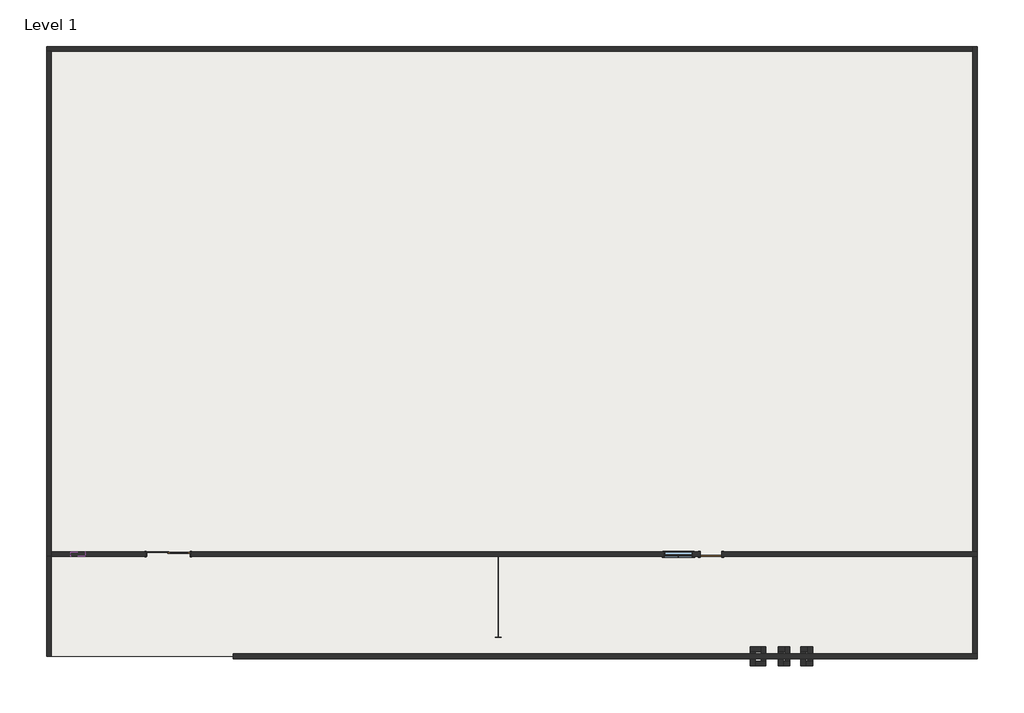
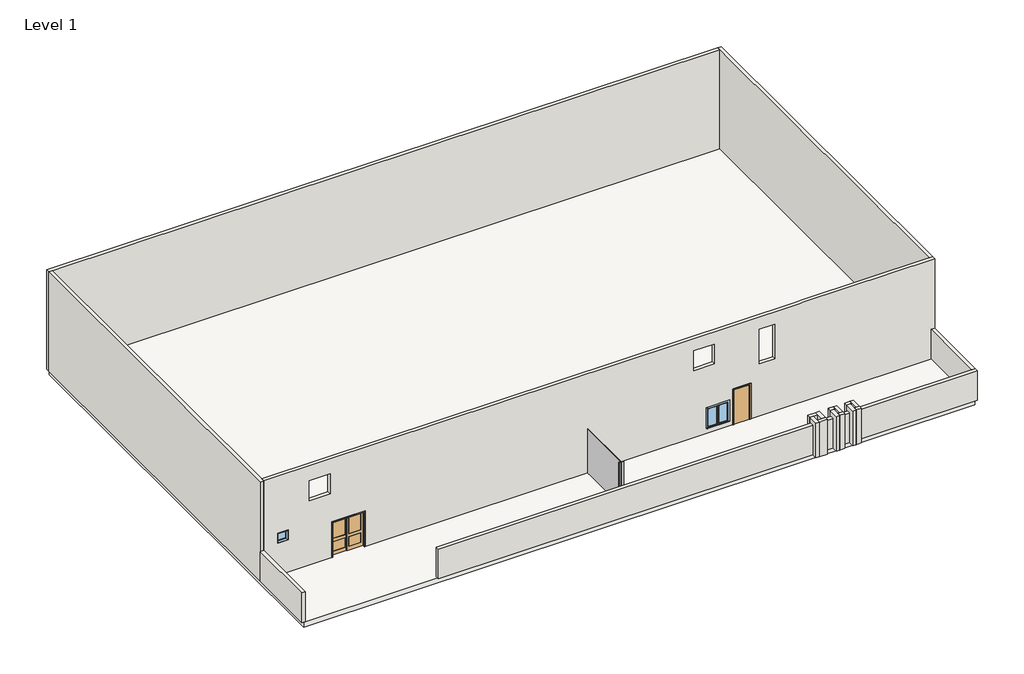
# One storey: 19 walls, 2 doors, 2 windows, 1 column, 1 slab.
"""IFC4 building model written with IfcOpenShell, lengths in millimetres."""

from ifc_helpers import new_model, si_unit, frame, origin, origin_with_axes, place, context, project, spatial, polyline, outline, extrude, faceted_brep, transform, mapped, element, save
from components import w_shapes_column_w10x49_8dea7e6f, door_6868039c, door_54dd4da4, window_0862ab64, window_6846e476

model = new_model("IFC4")

# Units and contexts
model_context = context("Model", 3, world=origin())
ifc_project = project(units=[si_unit("LENGTHUNIT", "METRE", prefix="MILLI")], contexts=[model_context])

# Site, building, storey
site = spatial("IfcSite", under=ifc_project)
building = spatial("IfcBuilding", under=site)
storey = spatial("IfcBuildingStorey", under=building, Name="Level 1", Elevation=0.0)

# Column
placement = place(None, origin())
w_shapes_column_w10x49_shape = w_shapes_column_w10x49_8dea7e6f(model_context)
element("IfcColumn", 1, ObjectType="W Shapes-Column : W10X49", at=placement, inside=storey, context=model_context, shape_type="MappedRepresentation", body=[
    mapped(w_shapes_column_w10x49_shape, transform((-3499.1858676, -16576.9422847, 0.0), x_axis=(1.0, 0.0, 0.0), y_axis=(0.0, 1.0, 0.0), z_axis=(0.0, 0.0, 1.0))),
])

# Doors
door_shape = door_6868039c(model_context)
element("IfcDoor", 2, ObjectType="Door-Interior-Double-Sliding-2_Panel-Wood : 72\" x 84\"", at=placement, inside=storey, context=model_context, shape_type="MappedRepresentation", body=[
    mapped(door_shape, transform((-17399.3252602, -14815.695124, 0.0), x_axis=(1.0, 0.0, 0.0), y_axis=(0.0, 1.0, 0.0), z_axis=(0.0, 0.0, 1.0))),
])
door_2_shape = door_54dd4da4(model_context)
element("IfcDoor", 3, ObjectType="Single-Flush : 36\" x 84\"", at=placement, inside=storey, context=model_context, shape_type="MappedRepresentation", body=[
    mapped(door_2_shape, transform((5460.6747398, -14818.870124, 0.0), x_axis=(-1.0, 0.0, 0.0), y_axis=(0.0, -1.0, 0.0), z_axis=(0.0, 0.0, 1.0))),
])

# Slab
element("IfcSlab", 4, ObjectType="Generic - 12\"", at=placement, inside=storey, context=model_context, shape_type="SweptSolid", body=[
    extrude(outline(polyline([(16585.8747398, 6480.1537948), (16585.8747398, -19123.0462052), (-22428.5252602, -19123.0462052), (-22428.5252602, 6480.1537948), (16585.8747398, 6480.1537948)])), frame((0.0, 0.0, -304.8), z_axis=(0.0, 0.0, 1.0), x_axis=(1.0, 0.0, 0.0)), (0.0, 0.0, 1.0), 304.8),
])

# Walls
element("IfcWall", 5, ObjectType="Generic - 8\"", at=placement, inside=storey, context=model_context, shape_type="Brep", body=[
    faceted_brep([(-22530.1252602, 6378.5537948, 0.0), (-22326.9252602, 6378.5537948, 0.0), (16484.2747398, 6378.5537948, 0.0), (16484.2747398, 6378.5537948, 6096.0), (-22326.9252602, 6378.5537948, 6096.0), (-22530.1252602, 6378.5537948, 6096.0), (-22530.1252602, 6581.7537948, 0.0), (-22530.1252602, 6581.7537948, 6096.0), (16484.2747398, 6581.7537948, 6096.0), (16484.2747398, 6581.7537948, 0.0)], [[[0, 1, 2, 3, 4, 5]], [[6, 7, 8, 9]], [[2, 1, 0, 6, 9]], [[5, 4, 3, 8, 7]], [[0, 5, 7, 6]], [[3, 2, 9, 8]]]),
])
element("IfcWall", 6, ObjectType="Generic - 8\"", at=placement, inside=storey, context=model_context, shape_type="Brep", body=[
    faceted_brep([(-22326.9252602, -14920.470124, 6096.0), (-22326.9252602, -14920.470124, 1828.8), (-22326.9252602, -14920.470124, 0.0), (-22326.9252602, -14717.270124, 0.0), (-22326.9252602, 6378.5537948, 0.0), (-22326.9252602, 6378.5537948, 6096.0), (-22326.9252602, -14717.270124, 6096.0), (-22530.1252602, -14920.470124, 0.0), (-22530.1252602, -14920.470124, 1828.8), (-22530.1252602, -14920.470124, 6096.0), (-22530.1252602, 6378.5537948, 6096.0), (-22530.1252602, 6378.5537948, 0.0)], [[[0, 1, 2, 3, 4, 5, 6]], [[7, 8, 9, 10, 11]], [[4, 3, 2, 7, 11]], [[0, 6, 5, 10, 9]], [[5, 4, 11, 10]], [[0, 9, 8, 7, 2, 1]]]),
])
element("IfcWall", 7, ObjectType="Generic - 8\"", at=placement, inside=storey, context=model_context, shape_type="Brep", body=[
    faceted_brep([(-22326.9252602, -14717.270124, 6096.0), (8806.3760973, -14717.270124, 6096.0), (9009.5760973, -14717.270124, 6096.0), (16484.2747398, -14717.270124, 6096.0), (16687.4747398, -14717.270124, 6096.0), (16687.4747398, -14717.270124, 0.0), (16484.2747398, -14717.270124, 0.0), (5917.8747398, -14717.270124, 0.0), (5917.8747398, -14717.270124, 2133.6), (5003.4747398, -14717.270124, 2133.6), (5003.4747398, -14717.270124, 0.0), (-16459.5252602, -14717.270124, 0.0), (-16459.5252602, -14717.270124, 2159.0), (-18339.1252602, -14717.270124, 2159.0), (-18339.1252602, -14717.270124, 0.0), (-22326.9252602, -14717.270124, 0.0), (-19685.3252602, -14717.270124, 5185.1493756), (-19685.3252602, -14717.270124, 3965.9493756), (-18466.1252602, -14717.270124, 3965.9493756), (-18466.1252602, -14717.270124, 5185.1493756), (-20904.5252602, -14717.270124, 1976.5444437), (-20904.5252602, -14717.270124, 2586.1444437), (-21514.1252602, -14717.270124, 2586.1444437), (-21514.1252602, -14717.270124, 1976.5444437), (6476.6747398, -14717.270124, 3200.4), (7391.0747398, -14717.270124, 3200.4), (7391.0747398, -14717.270124, 5334.0), (6476.6747398, -14717.270124, 5334.0), (2666.6747398, -14717.270124, 5334.0), (2666.6747398, -14717.270124, 4114.8), (3885.8747398, -14717.270124, 4114.8), (3885.8747398, -14717.270124, 5334.0), (3479.4747398, -14717.270124, 1524.0), (3479.4747398, -14717.270124, 304.8), (4698.6747398, -14717.270124, 304.8), (4698.6747398, -14717.270124, 1524.0), (16687.4747398, -14920.470124, 6096.0), (9009.5760973, -14920.470124, 6096.0), (8806.3760973, -14920.470124, 6096.0), (-22326.9252602, -14920.470124, 6096.0), (-22326.9252602, -14920.470124, 0.0), (-18339.1252602, -14920.470124, 0.0), (-18339.1252602, -14920.470124, 2159.0), (-16459.5252602, -14920.470124, 2159.0), (-16459.5252602, -14920.470124, 0.0), (5003.4747398, -14920.470124, 0.0), (5003.4747398, -14920.470124, 2133.6), (5917.8747398, -14920.470124, 2133.6), (5917.8747398, -14920.470124, 0.0), (16484.2747398, -14920.470124, 0.0), (16687.4747398, -14920.470124, 0.0), (16687.4747398, -14920.470124, 1828.8), (-19685.3252602, -14920.470124, 3965.9493756), (-19685.3252602, -14920.470124, 5185.1493756), (-18466.1252602, -14920.470124, 5185.1493756), (-18466.1252602, -14920.470124, 3965.9493756), (-20904.5252602, -14920.470124, 2586.1444437), (-20904.5252602, -14920.470124, 1976.5444437), (-21514.1252602, -14920.470124, 1976.5444437), (-21514.1252602, -14920.470124, 2586.1444437), (7391.0747398, -14920.470124, 3200.4), (6476.6747398, -14920.470124, 3200.4), (6476.6747398, -14920.470124, 5334.0), (7391.0747398, -14920.470124, 5334.0), (2666.6747398, -14920.470124, 4114.8), (2666.6747398, -14920.470124, 5334.0), (3885.8747398, -14920.470124, 5334.0), (3885.8747398, -14920.470124, 4114.8), (3479.4747398, -14920.470124, 304.8), (3479.4747398, -14920.470124, 1524.0), (4698.6747398, -14920.470124, 1524.0), (4698.6747398, -14920.470124, 304.8)], [[[0, 1, 2, 3, 4, 5, 6, 7, 8, 9, 10, 11, 12, 13, 14, 15], [16, 17, 18, 19], [20, 21, 22, 23], [24, 25, 26, 27], [28, 29, 30, 31], [32, 33, 34, 35]], [[36, 37, 38, 39, 40, 41, 42, 43, 44, 45, 46, 47, 48, 49, 50, 51], [52, 53, 54, 55], [56, 57, 58, 59], [60, 61, 62, 63], [64, 65, 66, 67], [68, 69, 70, 71]], [[5, 50, 49, 48, 7, 6]], [[40, 15, 14, 41]], [[10, 45, 44, 11]], [[4, 3, 2, 1, 0, 39, 38, 37, 36]], [[17, 16, 53, 52]], [[18, 17, 52, 55]], [[19, 18, 55, 54]], [[16, 19, 54, 53]], [[57, 56, 21, 20]], [[58, 57, 20, 23]], [[59, 58, 23, 22]], [[56, 59, 22, 21]], [[4, 36, 51, 50, 5]], [[15, 40, 39, 0]], [[61, 60, 25, 24]], [[62, 61, 24, 27]], [[63, 62, 27, 26]], [[60, 63, 26, 25]], [[46, 45, 10, 9]], [[47, 46, 9, 8]], [[48, 47, 8, 7]], [[29, 28, 65, 64]], [[30, 29, 64, 67]], [[31, 30, 67, 66]], [[28, 31, 66, 65]], [[32, 69, 68, 33]], [[34, 71, 70, 35]], [[69, 32, 35, 70]], [[71, 34, 33, 68]], [[43, 12, 11, 44]], [[12, 43, 42, 13]], [[13, 42, 41, 14]]]),
])
element("IfcWall", 8, ObjectType="Generic - 8\"", at=placement, inside=storey, context=model_context, shape_type="Brep", body=[
    faceted_brep([(16484.2747398, 6581.7537948, 0.0), (16484.2747398, 6378.5537948, 0.0), (16484.2747398, -14717.270124, 0.0), (16484.2747398, -14717.270124, 6096.0), (16484.2747398, 6378.5537948, 6096.0), (16484.2747398, 6581.7537948, 6096.0), (16687.4747398, 6581.7537948, 0.0), (16687.4747398, 6581.7537948, 6096.0), (16687.4747398, -14717.270124, 6096.0), (16687.4747398, -14717.270124, 0.0)], [[[0, 1, 2, 3, 4, 5]], [[6, 7, 8, 9]], [[2, 1, 0, 6, 9]], [[5, 4, 3, 8, 7]], [[0, 5, 7, 6]], [[2, 9, 8, 3]]]),
])
element("IfcWall", 9, ObjectType="Generic - 8\"", at=placement, inside=storey, context=model_context, shape_type="Brep", body=[
    faceted_brep([(-14656.1252602, -19224.6462052, 0.0), (16687.4747398, -19224.6462052, 0.0), (16687.4747398, -19224.6462052, 1828.8), (-14656.1252602, -19224.6462052, 1828.8), (-14656.1252602, -19021.4462052, 0.0), (-14656.1252602, -19021.4462052, 1828.8), (16484.2747398, -19021.4462052, 1828.8), (16687.4747398, -19021.4462052, 1828.8), (16687.4747398, -19021.4462052, 0.0), (16484.2747398, -19021.4462052, 0.0)], [[[0, 1, 2, 3]], [[4, 5, 6, 7, 8, 9]], [[1, 0, 4, 9, 8]], [[3, 2, 7, 6, 5]], [[0, 3, 5, 4]], [[2, 1, 8, 7]]]),
])
element("IfcWall", 10, ObjectType="Generic - 8\"", at=placement, inside=storey, context=model_context, shape_type="SweptSolid", body=[
    extrude(outline(polyline([(16687.4747398, -14920.470124), (16687.4747398, -19021.4462052), (16484.2747398, -19021.4462052), (16484.2747398, -14920.470124), (16687.4747398, -14920.470124)])), origin_with_axes(), (0.0, 0.0, 1.0), 1828.8),
])
element("IfcWall", 11, ObjectType="Generic - 8\"", at=placement, inside=storey, context=model_context, shape_type="SweptSolid", body=[
    extrude(outline(polyline([(-22530.1252602, -19123.0462052), (-22530.1252602, -14920.470124), (-22326.9252602, -14920.470124), (-22326.9252602, -19123.0462052), (-22530.1252602, -19123.0462052)])), origin_with_axes(), (0.0, 0.0, 1.0), 1828.8),
])
element("IfcWall", 12, ObjectType="Generic - 8\"", at=placement, inside=storey, context=model_context, shape_type="Brep", body=[
    faceted_brep([(7114.0258949, -18925.912129, 0.0), (7317.2258949, -18925.912129, 0.0), (7571.2258949, -18925.912129, 0.0), (7571.2258949, -18925.912129, 2133.6), (7317.2258949, -18925.912129, 2133.6), (7114.0258949, -18925.912129, 2133.6), (7114.0258949, -18722.712129, 0.0), (7114.0258949, -18722.712129, 2133.6), (7571.2258949, -18722.712129, 2133.6), (7571.2258949, -18722.712129, 0.0)], [[[0, 1, 2, 3, 4, 5]], [[6, 7, 8, 9]], [[2, 1, 0, 6, 9]], [[5, 4, 3, 8, 7]], [[0, 5, 7, 6]], [[3, 2, 9, 8]]]),
])
element("IfcWall", 13, ObjectType="Generic - 8\"", at=placement, inside=storey, context=model_context, shape_type="Brep", body=[
    faceted_brep([(7317.2258949, -19535.512129, 0.0), (7317.2258949, -19332.312129, 0.0), (7317.2258949, -18925.912129, 0.0), (7317.2258949, -18925.912129, 2133.6), (7317.2258949, -19332.312129, 2133.6), (7317.2258949, -19535.512129, 2133.6), (7114.0258949, -19535.512129, 0.0), (7114.0258949, -19535.512129, 2133.6), (7114.0258949, -18925.912129, 2133.6), (7114.0258949, -18925.912129, 0.0)], [[[0, 1, 2, 3, 4, 5]], [[6, 7, 8, 9]], [[2, 1, 0, 6, 9]], [[5, 4, 3, 8, 7]], [[0, 5, 7, 6]], [[3, 2, 9, 8]]]),
])
element("IfcWall", 14, ObjectType="Generic - 8\"", at=placement, inside=storey, context=model_context, shape_type="Brep", body=[
    faceted_brep([(7774.4258949, -19332.312129, 0.0), (7571.2258949, -19332.312129, 0.0), (7317.2258949, -19332.312129, 0.0), (7317.2258949, -19332.312129, 2133.6), (7571.2258949, -19332.312129, 2133.6), (7774.4258949, -19332.312129, 2133.6), (7774.4258949, -19535.512129, 0.0), (7774.4258949, -19535.512129, 2133.6), (7317.2258949, -19535.512129, 2133.6), (7317.2258949, -19535.512129, 0.0)], [[[0, 1, 2, 3, 4, 5]], [[6, 7, 8, 9]], [[2, 1, 0, 6, 9]], [[5, 4, 3, 8, 7]], [[0, 5, 7, 6]], [[3, 2, 9, 8]]]),
])
element("IfcWall", 15, ObjectType="Generic - 8\"", at=placement, inside=storey, context=model_context, shape_type="Brep", body=[
    faceted_brep([(7571.2258949, -18722.712129, 0.0), (7571.2258949, -18925.912129, 0.0), (7571.2258949, -19332.312129, 0.0), (7571.2258949, -19332.312129, 2133.6), (7571.2258949, -18925.912129, 2133.6), (7571.2258949, -18722.712129, 2133.6), (7774.4258949, -18722.712129, 0.0), (7774.4258949, -18722.712129, 2133.6), (7774.4258949, -19332.312129, 2133.6), (7774.4258949, -19332.312129, 0.0)], [[[0, 1, 2, 3, 4, 5]], [[6, 7, 8, 9]], [[2, 1, 0, 6, 9]], [[5, 4, 3, 8, 7]], [[0, 5, 7, 6]], [[3, 2, 9, 8]]]),
])
element("IfcWall", 16, ObjectType="Generic - 8\"", at=placement, inside=storey, context=model_context, shape_type="Brep", body=[
    faceted_brep([(8293.5945132, -18925.912129, 0.0), (8496.7945132, -18925.912129, 0.0), (8581.6287107, -18925.912129, 0.0), (8581.6287107, -18925.912129, 2133.6), (8496.7945132, -18925.912129, 2133.6), (8293.5945132, -18925.912129, 2133.6), (8293.5945132, -18722.712129, 0.0), (8293.5945132, -18722.712129, 2133.6), (8581.6287107, -18722.712129, 2133.6), (8581.6287107, -18722.712129, 0.0)], [[[0, 1, 2, 3, 4, 5]], [[6, 7, 8, 9]], [[2, 1, 0, 6, 9]], [[5, 4, 3, 8, 7]], [[0, 5, 7, 6]], [[3, 2, 9, 8]]]),
])
element("IfcWall", 17, ObjectType="Generic - 8\"", at=placement, inside=storey, context=model_context, shape_type="Brep", body=[
    faceted_brep([(8496.7945132, -19535.512129, 0.0), (8496.7945132, -19332.312129, 0.0), (8496.7945132, -18925.912129, 0.0), (8496.7945132, -18925.912129, 2133.6), (8496.7945132, -19332.312129, 2133.6), (8496.7945132, -19535.512129, 2133.6), (8293.5945132, -19535.512129, 0.0), (8293.5945132, -19535.512129, 2133.6), (8293.5945132, -18925.912129, 2133.6), (8293.5945132, -18925.912129, 0.0)], [[[0, 1, 2, 3, 4, 5]], [[6, 7, 8, 9]], [[2, 1, 0, 6, 9]], [[5, 4, 3, 8, 7]], [[0, 5, 7, 6]], [[3, 2, 9, 8]]]),
])
element("IfcWall", 18, ObjectType="Generic - 8\"", at=placement, inside=storey, context=model_context, shape_type="Brep", body=[
    faceted_brep([(8784.8287107, -19332.312129, 0.0), (8581.6287107, -19332.312129, 0.0), (8496.7945132, -19332.312129, 0.0), (8496.7945132, -19332.312129, 2133.6), (8581.6287107, -19332.312129, 2133.6), (8784.8287107, -19332.312129, 2133.6), (8784.8287107, -19535.512129, 0.0), (8784.8287107, -19535.512129, 2133.6), (8496.7945132, -19535.512129, 2133.6), (8496.7945132, -19535.512129, 0.0)], [[[0, 1, 2, 3, 4, 5]], [[6, 7, 8, 9]], [[2, 1, 0, 6, 9]], [[5, 4, 3, 8, 7]], [[0, 5, 7, 6]], [[3, 2, 9, 8]]]),
])
element("IfcWall", 19, ObjectType="Generic - 8\"", at=placement, inside=storey, context=model_context, shape_type="Brep", body=[
    faceted_brep([(8581.6287107, -18722.712129, 0.0), (8581.6287107, -18925.912129, 0.0), (8581.6287107, -19332.312129, 0.0), (8581.6287107, -19332.312129, 2133.6), (8581.6287107, -18925.912129, 2133.6), (8581.6287107, -18722.712129, 2133.6), (8784.8287107, -18722.712129, 0.0), (8784.8287107, -18722.712129, 2133.6), (8784.8287107, -19332.312129, 2133.6), (8784.8287107, -19332.312129, 0.0)], [[[0, 1, 2, 3, 4, 5]], [[6, 7, 8, 9]], [[2, 1, 0, 6, 9]], [[5, 4, 3, 8, 7]], [[0, 5, 7, 6]], [[3, 2, 9, 8]]]),
])
element("IfcWall", 20, ObjectType="Generic - 8\"", at=placement, inside=storey, context=model_context, shape_type="Brep", body=[
    faceted_brep([(9253.7085049, -18925.912129, 0.0), (9456.9085049, -18925.912129, 0.0), (9541.7427024, -18925.912129, 0.0), (9541.7427024, -18925.912129, 2133.6), (9456.9085049, -18925.912129, 2133.6), (9253.7085049, -18925.912129, 2133.6), (9253.7085049, -18722.712129, 0.0), (9253.7085049, -18722.712129, 2133.6), (9541.7427024, -18722.712129, 2133.6), (9541.7427024, -18722.712129, 0.0)], [[[0, 1, 2, 3, 4, 5]], [[6, 7, 8, 9]], [[2, 1, 0, 6, 9]], [[5, 4, 3, 8, 7]], [[0, 5, 7, 6]], [[3, 2, 9, 8]]]),
])
element("IfcWall", 21, ObjectType="Generic - 8\"", at=placement, inside=storey, context=model_context, shape_type="Brep", body=[
    faceted_brep([(9456.9085049, -19535.512129, 0.0), (9456.9085049, -19332.312129, 0.0), (9456.9085049, -18925.912129, 0.0), (9456.9085049, -18925.912129, 2133.6), (9456.9085049, -19332.312129, 2133.6), (9456.9085049, -19535.512129, 2133.6), (9253.7085049, -19535.512129, 0.0), (9253.7085049, -19535.512129, 2133.6), (9253.7085049, -18925.912129, 2133.6), (9253.7085049, -18925.912129, 0.0)], [[[0, 1, 2, 3, 4, 5]], [[6, 7, 8, 9]], [[2, 1, 0, 6, 9]], [[5, 4, 3, 8, 7]], [[0, 5, 7, 6]], [[3, 2, 9, 8]]]),
])
element("IfcWall", 22, ObjectType="Generic - 8\"", at=placement, inside=storey, context=model_context, shape_type="Brep", body=[
    faceted_brep([(9744.9427024, -19332.312129, 0.0), (9541.7427024, -19332.312129, 0.0), (9456.9085049, -19332.312129, 0.0), (9456.9085049, -19332.312129, 2133.6), (9541.7427024, -19332.312129, 2133.6), (9744.9427024, -19332.312129, 2133.6), (9744.9427024, -19535.512129, 0.0), (9744.9427024, -19535.512129, 2133.6), (9456.9085049, -19535.512129, 2133.6), (9456.9085049, -19535.512129, 0.0)], [[[0, 1, 2, 3, 4, 5]], [[6, 7, 8, 9]], [[2, 1, 0, 6, 9]], [[5, 4, 3, 8, 7]], [[0, 5, 7, 6]], [[3, 2, 9, 8]]]),
])
element("IfcWall", 23, ObjectType="Generic - 8\"", at=placement, inside=storey, context=model_context, shape_type="Brep", body=[
    faceted_brep([(9541.7427024, -18722.712129, 0.0), (9541.7427024, -18925.912129, 0.0), (9541.7427024, -19332.312129, 0.0), (9541.7427024, -19332.312129, 2133.6), (9541.7427024, -18925.912129, 2133.6), (9541.7427024, -18722.712129, 2133.6), (9744.9427024, -18722.712129, 0.0), (9744.9427024, -18722.712129, 2133.6), (9744.9427024, -19332.312129, 2133.6), (9744.9427024, -19332.312129, 0.0)], [[[0, 1, 2, 3, 4, 5]], [[6, 7, 8, 9]], [[2, 1, 0, 6, 9]], [[5, 4, 3, 8, 7]], [[0, 5, 7, 6]], [[3, 2, 9, 8]]]),
])

# Windows
window_shape = window_0862ab64(model_context)
element("IfcWindow", 24, ObjectType="Casement Dbl with Trim : 48\" x 48\"", at=placement, inside=storey, context=model_context, shape_type="MappedRepresentation", body=[
    mapped(window_shape, transform((4089.0747398, -14799.820124, -609.6), x_axis=(-1.0, 0.0, 0.0), y_axis=(0.0, -1.0, 0.0), z_axis=(0.0, 0.0, 1.0))),
])
window_2_shape = window_6846e476(model_context)
element("IfcWindow", 25, ObjectType="Fixed : 24\" x 24\"", at=placement, inside=storey, context=model_context, shape_type="MappedRepresentation", body=[
    mapped(window_2_shape, transform((-21171.2252602, -14818.870124, 1062.1444437), x_axis=(1.0, 0.0, 0.0), y_axis=(0.0, 1.0, 0.0), z_axis=(0.0, 0.0, 1.0))),
])

save(model, "model.ifc")

# Revit data of these elements
# Type "W Shapes-Column : W10X49"
#   Section Name Key = "W10x49"
#   Assembly Code = "B10"
#   Width = 10.000"
#   Web Thickness = 0.340"
#   Web Fillet = 0.500"
#   Warping Constant = 2070.00 in⁶
#   Torsional Moment of Inertia = 1.39 in⁴
#   Section Area = 14.40 in²
#   Plastic Modulus weak axis = 28.30 in³
#   Plastic Modulus strong axis = 60.40 in³
#   Perimeter = 58.50 ft²/ft
#   Nominal Weight = 49.00 lbf/ft
#   Moment of Inertia weak axis = 93.40 in⁴
#   Moment of Inertia strong axis = 272.00 in⁴
#   Height = 138.000"
#   Flange Thickness = 0.560"
#   Elastic Modulus weak axis = 18.70 in³
#   Elastic Modulus strong axis = 54.60 in³
#   Centroid Vertical = 69.000"
#   Centroid Horizontal = 5.000"
#   Structural Material [instance default] = Steel ASTM A992
#   Principal Axes Angle = 0
# Type "Door-Interior-Double-Sliding-2_Panel-Wood : 72\" x 84\""
#   Type Mark = "8"
#   Assembly Code = "C1020300"
#   Analytic Construction = "Wooden"
#   Top Rail = 0' - 4 11/16"
#   Thickness = 0' - 1 3/8"
#   Thermal Resistance (R) = 2.5876 (h·ft²·°F)/BTU
#   Stiles = 0' - 4 3/4"
#   Rough Width = 6' - 2"
#   Rough Height = 7' - 1"
#   Lock Rail = 0' - 7 1/2"
#   Height = 7' - 0"
#   Width = 6' - 0"
#   Heat Transfer Coefficient (U) = 0.3865 BTU/(h·ft²·°F)
#   Bottom Rail = 0' - 9 1/8"
#   Trim Material = Cherry
#   Panel Material = Cherry
#   Frame Material = Cherry
#   Visual Light Transmittance = 0
#   Solar Heat Gain Coefficient = 0
#   Wall Closure = (empty or 0)
#   Function = (empty or 0)
# Type "Single-Flush : 36\" x 84\""
#   Type Mark = "1"
#   Construction Type Id = "MDOOR"
#   Assembly Code = "C1020"
#   Analytic Construction = "Metal"
#   Thickness = 0' - 2"
#   Heat Transfer Coefficient (U) = 0.651978 BTU/(h·ft²·°F)
#   Height = 7' - 0"
#   Trim Projection Ext = 0' - 1"
#   Trim Projection Int = 0' - 1"
#   Trim Width = 0' - 3"
#   Width = 3' - 0"
#   Define Thermal Properties by = 1
#   Door Material = Door - Panel
#   Frame Material = Door - Frame
#   Visual Light Transmittance = 0
#   Solar Heat Gain Coefficient = 0
#   Function = (empty or 0)
#   Wall Closure = (empty or 0)
# Type "Generic - 12\""
#   Assembly Code = "B1010"
#   Function = 0
#   Layers, outside or top first: 1' - 0" no material (function 1)
# Type "Generic - 8\""
#   Assembly Code = "B2010"
#   Layers, outside or top first: 0' - 8" no material (function 1)
# Type "Casement Dbl with Trim : 48\" x 48\""
#   Type Mark = "10"
#   Construction Type Id = "GSP4R"
#   Assembly Code = "B2020100"
#   Analytic Construction = "1/8 in Pilkington single glazing"
#   Visual Light Transmittance = 0.9
#   Solar Heat Gain Coefficient = 0.78
#   Heat Transfer Coefficient (U) = 0.6496 BTU/(h·ft²·°F)
#   Height = 4' - 0"
#   Default Sill Height = 3' - 0"
#   Trim Projection - Ext. = 0' - 0 1/2"
#   Trim Projection - Int. = 0' - 0 3/4"
#   Trim Width - Exterior = 0' - 3 1/2"
#   Trim Width - Interior = 0' - 3 1/2"
#   Width = 4' - 0"
#   Window Inset = 0' - 0 3/4"
#   Define Thermal Properties by = 1
#   Glass Pane Material = Glass
#   Sash Material = Glass
#   Trim Exterior Material = Glass, Clear Glazing
#   Trim Interior Material = Trim
#   Wall Closure = (empty or 0)
# Type "Fixed : 24\" x 24\""
#   Type Mark = "3"
#   Construction Type Id = "GSP4R"
#   Assembly Code = "B2020100"
#   Analytic Construction = "1/8 in Pilkington single glazing"
#   Visual Light Transmittance = 0.9
#   Solar Heat Gain Coefficient = 0.78
#   Heat Transfer Coefficient (U) = 0.6496 BTU/(h·ft²·°F)
#   Height = 2' - 0"
#   Default Sill Height = 3' - 0"
#   Width = 2' - 0"
#   Window Inset = 0' - 0 3/4"
#   Define Thermal Properties by = 1
#   Glass Pane Material = Glass
#   Sash Material = Sash
#   Wall Closure = (empty or 0)
# Element 1 (IfcColumn, "W Shapes-Column : W10X49")
#   Structural Material = Steel ASTM A992
#   Phase Created = New Construction
#   Materials on its faces: "Steel ASTM A992"
# Element 2 (IfcDoor, "Door-Interior-Double-Sliding-2_Panel-Wood : 72\" x 84\"")
#   Phase Created = New Construction
#   Materials on its faces: "Cherry"
# Element 3 (IfcDoor, "Single-Flush : 36\" x 84\"")
#   Phase Created = New Construction
#   Materials on its faces: "Door - Frame", "Door - Panel"
# Element 4 (IfcSlab, "Generic - 12\"")
#   Height Offset From Level = 0' - 0"
#   Phase Created = New Construction
#   Materials on its faces: "Default Floor"
# Elements 5, 6, 7, 8 (IfcWall, "Generic - 8\"")
#   Top Offset = 0' - 0"
#   Base Offset = 0' - 0"
#   Unconnected Height = 20' - 0"
#   wall height = 20' - 0"
#   Phase Created = New Construction
#   Base Constraint = Level 1
#   Materials on its faces: "Default Wall"
# Elements 9, 10, 11 (IfcWall, "Generic - 8\"")
#   Top Offset = 0' - 0"
#   Base Offset = 0' - 0"
#   Unconnected Height = 6' - 0"
#   wall height = 6' - 0"
#   Phase Created = New Construction
#   Base Constraint = Level 1
#   Materials on its faces: "Default Wall"
# Elements 12, 13, 14, 15, 16, 17, 18, 19, 20, 21, 22, 23 (IfcWall, "Generic - 8\"")
#   Top Offset = 0' - 0"
#   Base Offset = 0' - 0"
#   Unconnected Height = 7' - 0"
#   wall height = 7' - 0"
#   Phase Created = New Construction
#   Base Constraint = Level 1
#   Materials on its faces: "Default Wall"
# Element 24 (IfcWindow, "Casement Dbl with Trim : 48\" x 48\"")
#   Mark = "9"
#   Phase Created = New Construction
#   Materials on its faces: "Glass", "Glass, Clear Glazing", "Trim"
# Element 25 (IfcWindow, "Fixed : 24\" x 24\"")
#   Mark = "2"
#   Phase Created = New Construction
#   Materials on its faces: "Sash", "Glass"
# Materials
#   "Steel ASTM A992": class "Metal", colour RGB 199 199 199, transparency 0, Description = "Structural steel 50ksi", Cost = 0
#   "Cherry": class "Wood", colour RGB 226 177 128, transparency 0, Description = "Prunus Serotina", Cost = 0
#   "Door - Panel": class "Wood", colour RGB 210 159 95, transparency 0
#   "Door - Frame": colour RGB 118 70 51, transparency 0
#   "Glass": class "Glass", colour RGB 0 128 192, transparency 0.75, Description = "Soda Lime Glass", Cost = 0
#   "Glass, Clear Glazing": class "Glass", colour RGB 0 128 192, transparency 0.75, Description = "Clear glazing", Cost = 0
#   "Trim": class "Wood", colour RGB 224 178 126, transparency 0
#   "Sash": class "Wood", colour RGB 224 178 126, transparency 0
#   "Default Floor": colour RGB 128 128 128, transparency 0
#   "Default Wall": colour RGB 128 128 128, transparency 0
